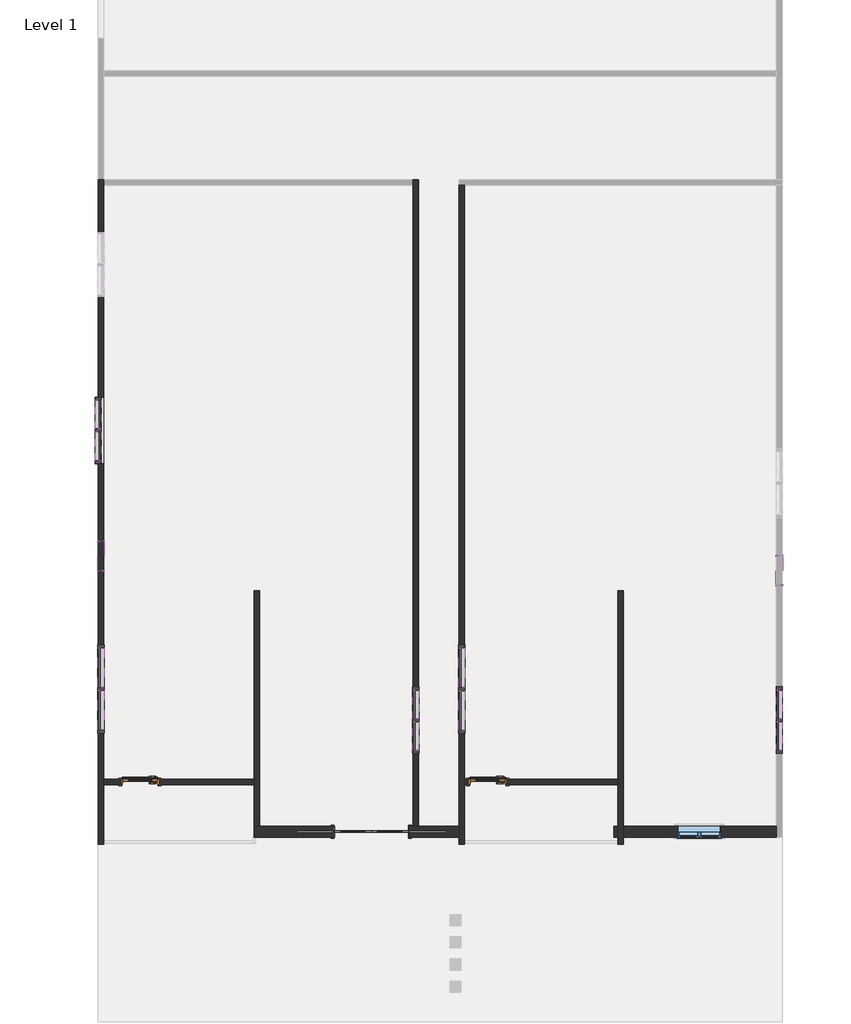
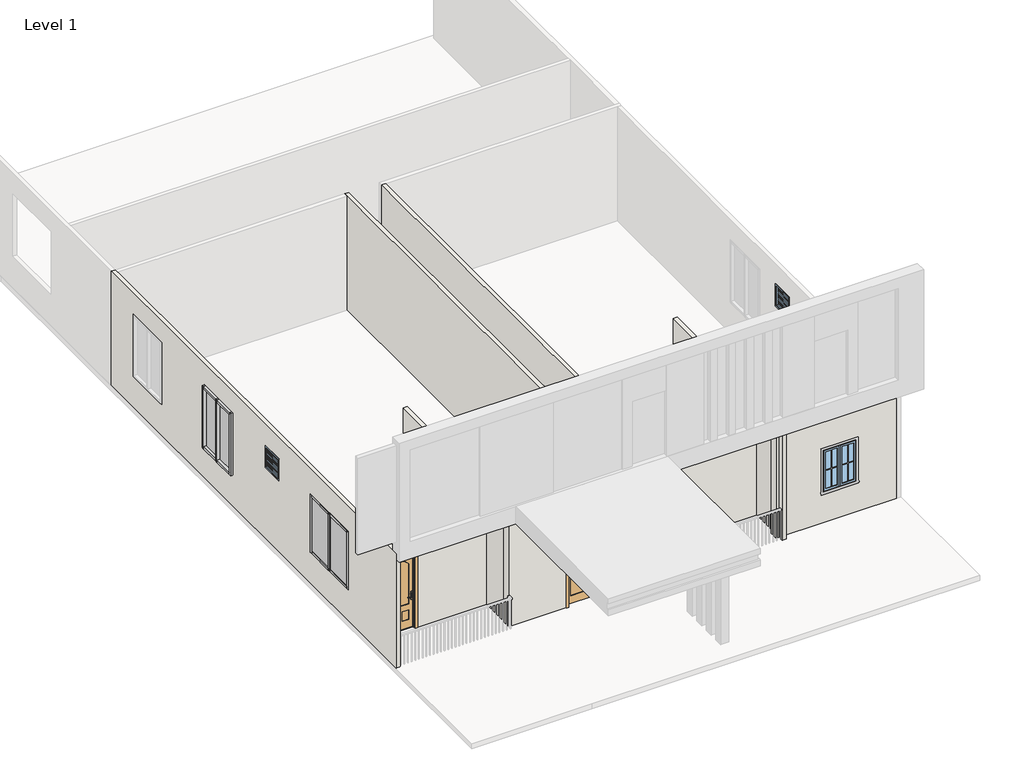
# One storey, part 1 of 3: 35 members, 10 plates, 9 walls, 3 doors, 3 windows.
"""IFC4 building model written with IfcOpenShell, lengths in millimetres."""

from ifc_helpers import new_model, si_unit, frame, origin, place, context, project, spatial, polyline, outline, extrude, faceted_brep, transform, mapped, element, save
from components import door_b81be692, door_7a66d0d1, member_8acf8d94, member_501b078b, member_2e6d4a6b, member_96ae0c19, member_d60e8053, member_2fae0574, member_b8ac15de, member_17644e48, system_panel_glazed_c4393626, system_panel_glazed_0e71bc1b, system_panel_glazed_e97abd02, system_panel_glazed_a7ecbca6, window_d341e8ac, window_d39e7ecb

model = new_model("IFC4")

# Units and contexts
model_context = context("Model", 3, world=origin())
ifc_project = project(units=[si_unit("LENGTHUNIT", "METRE", prefix="MILLI")], contexts=[model_context])

# Site, building, storey
site = spatial("IfcSite", under=ifc_project)
building = spatial("IfcBuilding", under=site)
storey = spatial("IfcBuildingStorey", under=building, Name="Level 1", Elevation=0.0)

# Doors
placement = place(None, origin())
door_shape = door_b81be692(model_context)
element("IfcDoor", 1, ObjectType="29\" x 84\"", at=placement, inside=storey, context=model_context, shape_type="MappedRepresentation", body=[
    mapped(door_shape, transform((-7346.707583, -9448.7163489, 0.0), x_axis=(1.0, 0.0, 0.0), y_axis=(0.0, 1.0, 0.0), z_axis=(0.0, 0.0, 1.0))),
])
element("IfcDoor", 2, ObjectType="29\" x 84\"", at=placement, inside=storey, context=model_context, shape_type="MappedRepresentation", body=[
    mapped(door_shape, transform((-172.2931282, -9448.9038009, 0.0), x_axis=(1.0, 0.0, 0.0), y_axis=(0.0, 1.0, 0.0), z_axis=(0.0, 0.0, 1.0))),
])
door_2_shape = door_7a66d0d1(model_context)
element("IfcDoor", 3, ObjectType="Door-Interior-Double-Pocket-2_Panel-Wood : 60\" x 84\"", at=placement, inside=storey, context=model_context, shape_type="MappedRepresentation", body=[
    mapped(door_2_shape, transform((-2570.8435762, -10471.5779557, 0.0), x_axis=(-1.0, 0.0, 0.0), y_axis=(0.0, -1.0, 0.0), z_axis=(0.0, 0.0, 1.0))),
])

# Members
member_shape = member_8acf8d94(model_context)
element("IfcMember", 4, ObjectType="Rectangular Mullion : 2.5\" x 5\" rectangular", at=placement, inside=storey, context=model_context, shape_type="MappedRepresentation", body=[
    mapped(member_shape, transform((-8153.157583, -8377.1401329, 2621.886558), x_axis=(0.0, 0.0, 1.0), y_axis=(-1.0, 0.0, 0.0), z_axis=(0.0, -1.0, 0.0))),
])
element("IfcMember", 5, ObjectType="Rectangular Mullion : 2.5\" x 5\" rectangular", at=placement, inside=storey, context=model_context, shape_type="MappedRepresentation", body=[
    mapped(member_shape, transform((-8153.157583, -7497.6651329, 2621.886558), x_axis=(0.0, 0.0, 1.0), y_axis=(-1.0, 0.0, 0.0), z_axis=(0.0, -1.0, 0.0))),
])
element("IfcMember", 6, ObjectType="Rectangular Mullion : 2.5\" x 5\" rectangular", at=placement, inside=storey, context=model_context, shape_type="MappedRepresentation", body=[
    mapped(member_shape, transform((-8153.157583, -6681.6901329, 914.4), x_axis=(0.0, 0.0, -1.0), y_axis=(-1.0, 0.0, 0.0), z_axis=(0.0, 1.0, 0.0))),
])
element("IfcMember", 7, ObjectType="Rectangular Mullion : 2.5\" x 5\" rectangular", at=placement, inside=storey, context=model_context, shape_type="MappedRepresentation", body=[
    mapped(member_shape, transform((-8153.157583, -7561.1651329, 914.4), x_axis=(0.0, 0.0, -1.0), y_axis=(-1.0, 0.0, 0.0), z_axis=(0.0, 1.0, 0.0))),
])
member_2_shape = member_501b078b(model_context)
element("IfcMember", 8, ObjectType="Rectangular Mullion : 2.5\" x 5\" rectangular", at=placement, inside=storey, context=model_context, shape_type="MappedRepresentation", body=[
    mapped(member_2_shape, transform((5848.1708786, -8795.0998253, 2743.2), x_axis=(0.0, 0.0, 1.0), y_axis=(-1.0, 0.0, 0.0), z_axis=(0.0, -1.0, 0.0))),
])
element("IfcMember", 9, ObjectType="Rectangular Mullion : 2.5\" x 5\" rectangular", at=placement, inside=storey, context=model_context, shape_type="MappedRepresentation", body=[
    mapped(member_2_shape, transform((5848.1708786, -8142.1745373, 2743.2), x_axis=(0.0, 0.0, 1.0), y_axis=(-1.0, 0.0, 0.0), z_axis=(0.0, -1.0, 0.0))),
])
element("IfcMember", 10, ObjectType="Rectangular Mullion : 2.5\" x 5\" rectangular", at=placement, inside=storey, context=model_context, shape_type="MappedRepresentation", body=[
    mapped(member_2_shape, transform((-1656.4435762, -8795.0998253, 2743.2), x_axis=(0.0, 0.0, 1.0), y_axis=(-1.0, 0.0, 0.0), z_axis=(0.0, -1.0, 0.0))),
])
element("IfcMember", 11, ObjectType="Rectangular Mullion : 2.5\" x 5\" rectangular", at=placement, inside=storey, context=model_context, shape_type="MappedRepresentation", body=[
    mapped(member_2_shape, transform((-1656.4435762, -8142.1745373, 2743.2), x_axis=(0.0, 0.0, 1.0), y_axis=(-1.0, 0.0, 0.0), z_axis=(0.0, -1.0, 0.0))),
])
element("IfcMember", 12, ObjectType="Rectangular Mullion : 2.5\" x 5\" rectangular", at=placement, inside=storey, context=model_context, shape_type="MappedRepresentation", body=[
    mapped(member_2_shape, transform((5848.1708786, -7552.7492493, 914.4), x_axis=(0.0, 0.0, -1.0), y_axis=(-1.0, 0.0, 0.0), z_axis=(0.0, 1.0, 0.0))),
])
element("IfcMember", 13, ObjectType="Rectangular Mullion : 2.5\" x 5\" rectangular", at=placement, inside=storey, context=model_context, shape_type="MappedRepresentation", body=[
    mapped(member_2_shape, transform((5848.1708786, -8205.6745373, 914.4), x_axis=(0.0, 0.0, -1.0), y_axis=(-1.0, 0.0, 0.0), z_axis=(0.0, 1.0, 0.0))),
])
element("IfcMember", 14, ObjectType="Rectangular Mullion : 2.5\" x 5\" rectangular", at=placement, inside=storey, context=model_context, shape_type="MappedRepresentation", body=[
    mapped(member_2_shape, transform((-1656.4435762, -7552.7492493, 914.4), x_axis=(0.0, 0.0, -1.0), y_axis=(-1.0, 0.0, 0.0), z_axis=(0.0, 1.0, 0.0))),
])
element("IfcMember", 15, ObjectType="Rectangular Mullion : 2.5\" x 5\" rectangular", at=placement, inside=storey, context=model_context, shape_type="MappedRepresentation", body=[
    mapped(member_2_shape, transform((-1656.4435762, -8205.6745373, 914.4), x_axis=(0.0, 0.0, -1.0), y_axis=(-1.0, 0.0, 0.0), z_axis=(0.0, 1.0, 0.0))),
])
member_3_shape = member_2e6d4a6b(model_context)
element("IfcMember", 16, ObjectType="Rectangular Mullion : 2.5\" x 5\" rectangular", at=placement, inside=storey, context=model_context, shape_type="MappedRepresentation", body=[
    mapped(member_3_shape, transform((-705.6931282, -8380.4909009, 2743.2), x_axis=(0.0, 0.0, 1.0), y_axis=(-1.0, 0.0, 0.0), z_axis=(0.0, -1.0, 0.0))),
])
element("IfcMember", 17, ObjectType="Rectangular Mullion : 2.5\" x 5\" rectangular", at=placement, inside=storey, context=model_context, shape_type="MappedRepresentation", body=[
    mapped(member_3_shape, transform((-705.6931282, -7499.3405169, 2743.2), x_axis=(0.0, 0.0, 1.0), y_axis=(-1.0, 0.0, 0.0), z_axis=(0.0, -1.0, 0.0))),
])
element("IfcMember", 18, ObjectType="Rectangular Mullion : 2.5\" x 5\" rectangular", at=placement, inside=storey, context=model_context, shape_type="MappedRepresentation", body=[
    mapped(member_3_shape, transform((-705.6931282, -6681.6901329, 914.4), x_axis=(0.0, 0.0, -1.0), y_axis=(-1.0, 0.0, 0.0), z_axis=(0.0, 1.0, 0.0))),
])
element("IfcMember", 19, ObjectType="Rectangular Mullion : 2.5\" x 5\" rectangular", at=placement, inside=storey, context=model_context, shape_type="MappedRepresentation", body=[
    mapped(member_3_shape, transform((-705.6931282, -7562.8405169, 914.4), x_axis=(0.0, 0.0, -1.0), y_axis=(-1.0, 0.0, 0.0), z_axis=(0.0, 1.0, 0.0))),
])
member_4_shape = member_96ae0c19(model_context)
element("IfcMember", 20, ObjectType="Rectangular Mullion : 2.5\" x 5\" rectangular", at=placement, inside=storey, context=model_context, shape_type="MappedRepresentation", body=[
    mapped(member_4_shape, transform((-8210.307583, -2819.4060617, 2743.2), x_axis=(0.0, 0.0, 1.0), y_axis=(-1.0, 0.0, 0.0), z_axis=(0.0, -1.0, 0.0))),
])
element("IfcMember", 21, ObjectType="Rectangular Mullion : 2.5\" x 5\" rectangular", at=placement, inside=storey, context=model_context, shape_type="MappedRepresentation", body=[
    mapped(member_4_shape, transform((-8210.307583, -2164.5788979, 2743.2), x_axis=(0.0, 0.0, 1.0), y_axis=(-1.0, 0.0, 0.0), z_axis=(0.0, -1.0, 0.0))),
])
element("IfcMember", 22, ObjectType="Rectangular Mullion : 2.5\" x 5\" rectangular", at=placement, inside=storey, context=model_context, shape_type="MappedRepresentation", body=[
    mapped(member_4_shape, transform((-8210.307583, -1573.2517341, 914.4), x_axis=(0.0, 0.0, -1.0), y_axis=(-1.0, 0.0, 0.0), z_axis=(0.0, 1.0, 0.0))),
])
element("IfcMember", 23, ObjectType="Rectangular Mullion : 2.5\" x 5\" rectangular", at=placement, inside=storey, context=model_context, shape_type="MappedRepresentation", body=[
    mapped(member_4_shape, transform((-8210.307583, -2228.0788979, 914.4), x_axis=(0.0, 0.0, -1.0), y_axis=(-1.0, 0.0, 0.0), z_axis=(0.0, 1.0, 0.0))),
])
member_5_shape = member_d60e8053(model_context)
element("IfcMember", 24, ObjectType="Rectangular Mullion : 2.5\" x 5\" rectangular", at=placement, inside=storey, context=model_context, shape_type="MappedRepresentation", body=[
    mapped(member_5_shape, transform((-8210.307583, -2196.3288979, 914.4), x_axis=(0.0, -1.0, 0.0), y_axis=(-1.0, 0.0, 0.0), z_axis=(0.0, 0.0, -1.0))),
])
member_6_shape = member_2fae0574(model_context)
element("IfcMember", 25, ObjectType="Rectangular Mullion : 2.5\" x 5\" rectangular", at=placement, inside=storey, context=model_context, shape_type="MappedRepresentation", body=[
    mapped(member_6_shape, transform((-8210.307583, -1509.7517341, 2743.2), x_axis=(0.0, 1.0, 0.0), y_axis=(-1.0, 0.0, 0.0), z_axis=(0.0, 0.0, 1.0))),
])
element("IfcMember", 26, ObjectType="Rectangular Mullion : 2.5\" x 5\" rectangular", at=placement, inside=storey, context=model_context, shape_type="MappedRepresentation", body=[
    mapped(member_6_shape, transform((-8210.307583, -2882.9060617, 914.4), x_axis=(0.0, -1.0, 0.0), y_axis=(-1.0, 0.0, 0.0), z_axis=(0.0, 0.0, -1.0))),
])
member_7_shape = member_b8ac15de(model_context)
element("IfcMember", 27, ObjectType="Rectangular Mullion : 2.5\" x 5\" rectangular", at=placement, inside=storey, context=model_context, shape_type="MappedRepresentation", body=[
    mapped(member_7_shape, transform((-8153.157583, -7529.4151329, 914.4), x_axis=(0.0, -1.0, 0.0), y_axis=(-1.0, 0.0, 0.0), z_axis=(0.0, 0.0, -1.0))),
])
member_8_shape = member_17644e48(model_context)
element("IfcMember", 28, ObjectType="Rectangular Mullion : 2.5\" x 5\" rectangular", at=placement, inside=storey, context=model_context, shape_type="MappedRepresentation", body=[
    mapped(member_8_shape, transform((-8153.157583, -6618.1901329, 2621.886558), x_axis=(0.0, 1.0, 0.0), y_axis=(-1.0, 0.0, 0.0), z_axis=(0.0, 0.0, 1.0))),
])
element("IfcMember", 29, ObjectType="Rectangular Mullion : 2.5\" x 5\" rectangular", at=placement, inside=storey, context=model_context, shape_type="MappedRepresentation", body=[
    mapped(member_8_shape, transform((-8153.157583, -8440.6401329, 914.4), x_axis=(0.0, -1.0, 0.0), y_axis=(-1.0, 0.0, 0.0), z_axis=(0.0, 0.0, -1.0))),
])
element("IfcMember", 30, ObjectType="Rectangular Mullion : 2.5\" x 5\" rectangular", at=placement, inside=storey, context=model_context, shape_type="MappedRepresentation", body=[
    mapped(member_5_shape, transform((5848.1708786, -8173.9245373, 914.4), x_axis=(0.0, -1.0, 0.0), y_axis=(-1.0, 0.0, 0.0), z_axis=(0.0, 0.0, -1.0))),
])
element("IfcMember", 31, ObjectType="Rectangular Mullion : 2.5\" x 5\" rectangular", at=placement, inside=storey, context=model_context, shape_type="MappedRepresentation", body=[
    mapped(member_5_shape, transform((-1656.4435762, -8173.9245373, 914.4), x_axis=(0.0, -1.0, 0.0), y_axis=(-1.0, 0.0, 0.0), z_axis=(0.0, 0.0, -1.0))),
])
element("IfcMember", 32, ObjectType="Rectangular Mullion : 2.5\" x 5\" rectangular", at=placement, inside=storey, context=model_context, shape_type="MappedRepresentation", body=[
    mapped(member_5_shape, transform((-705.6931282, -7531.0905169, 914.4), x_axis=(0.0, -1.0, 0.0), y_axis=(-1.0, 0.0, 0.0), z_axis=(0.0, 0.0, -1.0))),
])
element("IfcMember", 33, ObjectType="Rectangular Mullion : 2.5\" x 5\" rectangular", at=placement, inside=storey, context=model_context, shape_type="MappedRepresentation", body=[
    mapped(member_6_shape, transform((5848.1708786, -7489.2492493, 2743.2), x_axis=(0.0, 1.0, 0.0), y_axis=(-1.0, 0.0, 0.0), z_axis=(0.0, 0.0, 1.0))),
])
element("IfcMember", 34, ObjectType="Rectangular Mullion : 2.5\" x 5\" rectangular", at=placement, inside=storey, context=model_context, shape_type="MappedRepresentation", body=[
    mapped(member_6_shape, transform((-1656.4435762, -7489.2492493, 2743.2), x_axis=(0.0, 1.0, 0.0), y_axis=(-1.0, 0.0, 0.0), z_axis=(0.0, 0.0, 1.0))),
])
element("IfcMember", 35, ObjectType="Rectangular Mullion : 2.5\" x 5\" rectangular", at=placement, inside=storey, context=model_context, shape_type="MappedRepresentation", body=[
    mapped(member_6_shape, transform((-705.6931282, -6618.1901329, 2743.2), x_axis=(0.0, 1.0, 0.0), y_axis=(-1.0, 0.0, 0.0), z_axis=(0.0, 0.0, 1.0))),
])
element("IfcMember", 36, ObjectType="Rectangular Mullion : 2.5\" x 5\" rectangular", at=placement, inside=storey, context=model_context, shape_type="MappedRepresentation", body=[
    mapped(member_6_shape, transform((5848.1708786, -8858.5998253, 914.4), x_axis=(0.0, -1.0, 0.0), y_axis=(-1.0, 0.0, 0.0), z_axis=(0.0, 0.0, -1.0))),
])
element("IfcMember", 37, ObjectType="Rectangular Mullion : 2.5\" x 5\" rectangular", at=placement, inside=storey, context=model_context, shape_type="MappedRepresentation", body=[
    mapped(member_6_shape, transform((-1656.4435762, -8858.5998253, 914.4), x_axis=(0.0, -1.0, 0.0), y_axis=(-1.0, 0.0, 0.0), z_axis=(0.0, 0.0, -1.0))),
])
element("IfcMember", 38, ObjectType="Rectangular Mullion : 2.5\" x 5\" rectangular", at=placement, inside=storey, context=model_context, shape_type="MappedRepresentation", body=[
    mapped(member_6_shape, transform((-705.6931282, -8443.9909009, 914.4), x_axis=(0.0, -1.0, 0.0), y_axis=(-1.0, 0.0, 0.0), z_axis=(0.0, 0.0, -1.0))),
])

# Plates
system_panel_glazed_shape = system_panel_glazed_c4393626(model_context)
element("IfcPlate", 39, ObjectType="System Panel : Glazed", at=placement, inside=storey, context=model_context, shape_type="MappedRepresentation", body=[
    mapped(system_panel_glazed_shape, transform((-8210.307583, -1868.915316, 977.9), x_axis=(0.0, -1.0, 0.0), y_axis=(1.0, 0.0, 0.0), z_axis=(0.0, 0.0, 1.0))),
])
element("IfcPlate", 40, ObjectType="System Panel : Glazed", at=placement, inside=storey, context=model_context, shape_type="MappedRepresentation", body=[
    mapped(system_panel_glazed_shape, transform((-8210.307583, -2523.7424798, 977.9), x_axis=(0.0, -1.0, 0.0), y_axis=(1.0, 0.0, 0.0), z_axis=(0.0, 0.0, 1.0))),
])
system_panel_glazed_2_shape = system_panel_glazed_0e71bc1b(model_context)
element("IfcPlate", 41, ObjectType="System Panel : Glazed", at=placement, inside=storey, context=model_context, shape_type="MappedRepresentation", body=[
    mapped(system_panel_glazed_2_shape, transform((-8153.157583, -7089.6776329, 977.9), x_axis=(0.0, -1.0, 0.0), y_axis=(1.0, 0.0, 0.0), z_axis=(0.0, 0.0, 1.0))),
])
element("IfcPlate", 42, ObjectType="System Panel : Glazed", at=placement, inside=storey, context=model_context, shape_type="MappedRepresentation", body=[
    mapped(system_panel_glazed_2_shape, transform((-8153.157583, -7969.1526329, 977.9), x_axis=(0.0, -1.0, 0.0), y_axis=(1.0, 0.0, 0.0), z_axis=(0.0, 0.0, 1.0))),
])
system_panel_glazed_3_shape = system_panel_glazed_e97abd02(model_context)
element("IfcPlate", 43, ObjectType="System Panel : Glazed", at=placement, inside=storey, context=model_context, shape_type="MappedRepresentation", body=[
    mapped(system_panel_glazed_3_shape, transform((5848.1708786, -7847.4618933, 977.9), x_axis=(0.0, -1.0, 0.0), y_axis=(1.0, 0.0, 0.0), z_axis=(0.0, 0.0, 1.0))),
])
element("IfcPlate", 44, ObjectType="System Panel : Glazed", at=placement, inside=storey, context=model_context, shape_type="MappedRepresentation", body=[
    mapped(system_panel_glazed_3_shape, transform((-1656.4435762, -7847.4618933, 977.9), x_axis=(0.0, -1.0, 0.0), y_axis=(1.0, 0.0, 0.0), z_axis=(0.0, 0.0, 1.0))),
])
element("IfcPlate", 45, ObjectType="System Panel : Glazed", at=placement, inside=storey, context=model_context, shape_type="MappedRepresentation", body=[
    mapped(system_panel_glazed_3_shape, transform((5848.1708786, -8500.3871813, 977.9), x_axis=(0.0, -1.0, 0.0), y_axis=(1.0, 0.0, 0.0), z_axis=(0.0, 0.0, 1.0))),
])
element("IfcPlate", 46, ObjectType="System Panel : Glazed", at=placement, inside=storey, context=model_context, shape_type="MappedRepresentation", body=[
    mapped(system_panel_glazed_3_shape, transform((-1656.4435762, -8500.3871813, 977.9), x_axis=(0.0, -1.0, 0.0), y_axis=(1.0, 0.0, 0.0), z_axis=(0.0, 0.0, 1.0))),
])
system_panel_glazed_4_shape = system_panel_glazed_a7ecbca6(model_context)
element("IfcPlate", 47, ObjectType="System Panel : Glazed", at=placement, inside=storey, context=model_context, shape_type="MappedRepresentation", body=[
    mapped(system_panel_glazed_4_shape, transform((-705.6931282, -7090.5153249, 977.9), x_axis=(0.0, -1.0, 0.0), y_axis=(1.0, 0.0, 0.0), z_axis=(0.0, 0.0, 1.0))),
])
element("IfcPlate", 48, ObjectType="System Panel : Glazed", at=placement, inside=storey, context=model_context, shape_type="MappedRepresentation", body=[
    mapped(system_panel_glazed_4_shape, transform((-705.6931282, -7971.6657089, 977.9), x_axis=(0.0, -1.0, 0.0), y_axis=(1.0, 0.0, 0.0), z_axis=(0.0, 0.0, 1.0))),
])

# Walls
element("IfcWall", 49, ObjectType="4.5\" wall", at=placement, inside=storey, context=model_context, shape_type="Brep", body=[
    faceted_brep([(-8096.007583, -10738.0280197, 0.0), (-8096.007583, -9509.0413489, 0.0), (-8096.007583, -9394.7413489, 0.0), (-8096.007583, 2864.0002499, 0.0), (-8096.007583, 2978.3002499, 0.0), (-8096.007583, 2978.3002499, 3352.8), (-8096.007583, 2864.0002499, 3352.8), (-8096.007583, -9394.7413489, 3352.8), (-8096.007583, -9509.0413489, 3352.8), (-8096.007583, -10738.0280197, 3352.8), (-8096.007583, -6618.1901329, 2621.886558), (-8096.007583, -6618.1901329, 914.4), (-8096.007583, -8440.6401329, 914.4), (-8096.007583, -8440.6401329, 2621.886558), (-8096.007583, -5094.1901329, 2724.15), (-8096.007583, -4484.5901329, 2724.15), (-8096.007583, -4484.5901329, 2114.55), (-8096.007583, -5094.1901329, 2114.55), (-8096.007583, 1909.8209543, 2743.2), (-8096.007583, 1909.8209543, 914.4), (-8096.007583, 536.6666267, 914.4), (-8096.007583, 536.6666267, 2743.2), (-8096.007583, -1509.7517341, 2743.2), (-8096.007583, -1509.7517341, 914.4), (-8096.007583, -2882.9060617, 914.4), (-8096.007583, -2882.9060617, 2743.2), (-8210.307583, 2978.3002499, 0.0), (-8210.307583, -10738.0280197, 0.0), (-8210.307583, -10738.0280197, 3352.8), (-8210.307583, 2978.3002499, 3352.8), (-8210.307583, -6618.1901329, 914.4), (-8210.307583, -6618.1901329, 2621.886558), (-8210.307583, -8440.6401329, 2621.886558), (-8210.307583, -8440.6401329, 914.4), (-8210.307583, -5094.1901329, 2724.15), (-8210.307583, -5094.1901329, 2114.55), (-8210.307583, -4484.5901329, 2114.55), (-8210.307583, -4484.5901329, 2724.15), (-8210.307583, 1909.8209543, 914.4), (-8210.307583, 1909.8209543, 2743.2), (-8210.307583, 536.6666267, 2743.2), (-8210.307583, 536.6666267, 914.4), (-8210.307583, -1509.7517341, 914.4), (-8210.307583, -1509.7517341, 2743.2), (-8210.307583, -2882.9060617, 2743.2), (-8210.307583, -2882.9060617, 914.4)], [[[0, 1, 2, 3, 4, 5, 6, 7, 8, 9], [10, 11, 12, 13], [14, 15, 16, 17], [18, 19, 20, 21], [22, 23, 24, 25]], [[26, 27, 28, 29], [30, 31, 32, 33], [34, 35, 36, 37], [38, 39, 40, 41], [42, 43, 44, 45]], [[4, 3, 2, 1, 0, 27, 26]], [[9, 8, 7, 6, 5, 29, 28]], [[0, 9, 28, 27]], [[5, 4, 26, 29]], [[10, 31, 30, 11]], [[31, 10, 13, 32]], [[32, 13, 12, 33]], [[11, 30, 33, 12]], [[35, 34, 14, 17]], [[36, 35, 17, 16]], [[37, 36, 16, 15]], [[34, 37, 15, 14]], [[38, 19, 18, 39]], [[39, 18, 21, 40]], [[40, 21, 20, 41]], [[19, 38, 41, 20]], [[22, 43, 42, 23]], [[43, 22, 25, 44]], [[44, 25, 24, 45]], [[23, 42, 45, 24]]]),
])
element("IfcWall", 50, ObjectType="4.5\" wall", at=placement, inside=storey, context=model_context, shape_type="Brep", body=[
    faceted_brep([(-1599.2935762, -10357.2779557, 0.0), (-1599.2935762, 2978.3002499, 0.0), (-1599.2935762, 2978.3002499, 3352.8), (-1599.2935762, -10357.2779557, 3352.8), (-1599.2935762, -7489.2492493, 2743.2), (-1599.2935762, -7489.2492493, 914.4), (-1599.2935762, -8858.5998253, 914.4), (-1599.2935762, -8858.5998253, 2743.2), (-1713.5935762, 2978.3002499, 0.0), (-1713.5935762, 2864.0002499, 0.0), (-1713.5935762, -10357.2779557, 0.0), (-1713.5935762, -10357.2779557, 3352.8), (-1713.5935762, 2864.0002499, 3352.8), (-1713.5935762, 2978.3002499, 3352.8), (-1713.5935762, -7489.2492493, 914.4), (-1713.5935762, -7489.2492493, 2743.2), (-1713.5935762, -8858.5998253, 2743.2), (-1713.5935762, -8858.5998253, 914.4)], [[[0, 1, 2, 3], [4, 5, 6, 7]], [[8, 9, 10, 11, 12, 13], [14, 15, 16, 17]], [[1, 0, 10, 9, 8]], [[3, 2, 13, 12, 11]], [[2, 1, 8, 13]], [[0, 3, 11, 10]], [[14, 5, 4, 15]], [[15, 4, 7, 16]], [[16, 7, 6, 17]], [[5, 14, 17, 6]]]),
])
element("IfcWall", 51, ObjectType="4.5\" wall", at=placement, inside=storey, context=model_context, shape_type="Brep", body=[
    faceted_brep([(-762.8431282, 2864.0002499, 0.0), (-762.8431282, -10357.2779557, 0.0), (-762.8431282, -10450.9404557, 0.0), (-762.8431282, -10492.2154557, 0.0), (-762.8431282, -10585.8779557, 0.0), (-762.8431282, -10737.6531157, 0.0), (-762.8431282, -10737.6531157, 3352.8), (-762.8431282, -10585.8779557, 3352.8), (-762.8431282, -10357.2779557, 3352.8), (-762.8431282, 2864.0002499, 3352.8), (-762.8431282, -6618.1901329, 914.4), (-762.8431282, -6618.1901329, 2743.2), (-762.8431282, -8443.9909009, 2743.2), (-762.8431282, -8443.9909009, 914.4), (-648.5431282, -10737.6531157, 0.0), (-648.5431282, -9509.2288009, 0.0), (-648.5431282, -9394.9288009, 0.0), (-648.5431282, 2864.0002499, 0.0), (-648.5431282, 2864.0002499, 3352.8), (-648.5431282, -9394.9288009, 3352.8), (-648.5431282, -9509.2288009, 3352.8), (-648.5431282, -10737.6531157, 3352.8), (-648.5431282, -6618.1901329, 2743.2), (-648.5431282, -6618.1901329, 914.4), (-648.5431282, -8443.9909009, 914.4), (-648.5431282, -8443.9909009, 2743.2)], [[[0, 1, 2, 3, 4, 5, 6, 7, 8, 9], [10, 11, 12, 13]], [[14, 15, 16, 17, 18, 19, 20, 21], [22, 23, 24, 25]], [[5, 4, 3, 2, 1, 0, 17, 16, 15, 14]], [[6, 5, 14, 21]], [[9, 8, 7, 6, 21, 20, 19, 18]], [[0, 9, 18, 17]], [[10, 23, 22, 11]], [[11, 22, 25, 12]], [[12, 25, 24, 13]], [[23, 10, 13, 24]]]),
])
element("IfcWall", 52, ObjectType="4.5\" wall", at=placement, inside=storey, context=model_context, shape_type="Brep", body=[
    faceted_brep([(-4874.3237038, -10357.2779557, 0.0), (-4874.3237038, -5507.4946657, 0.0), (-4874.3237038, -5507.4946657, 3352.8), (-4874.3237038, -10357.2779557, 3352.8), (-4988.6237038, -10357.2779557, 0.0), (-4988.6237038, -10357.2779557, 3352.8), (-4988.6237038, -9509.0413489, 3352.8), (-4988.6237038, -9394.7413489, 3352.8), (-4988.6237038, -5507.4946657, 3352.8), (-4988.6237038, -5507.4946657, 0.0), (-4988.6237038, -9394.7413489, 0.0), (-4988.6237038, -9509.0413489, 0.0)], [[[0, 1, 2, 3]], [[4, 5, 6, 7, 8, 9, 10, 11]], [[1, 0, 4, 11, 10, 9]], [[2, 1, 9, 8]], [[3, 2, 8, 7, 6, 5]], [[0, 3, 5, 4]]]),
])
element("IfcWall", 53, ObjectType="4.5\" wall", at=placement, inside=storey, context=model_context, shape_type="Brep", body=[
    faceted_brep([(2515.990751, -5507.4946657, 0.0), (2515.990751, -9394.9288009, 0.0), (2515.990751, -9509.2288009, 0.0), (2515.990751, -10737.6531157, 0.0), (2515.990751, -10737.6531157, 3352.8), (2515.990751, -9509.2288009, 3352.8), (2515.990751, -9394.9288009, 3352.8), (2515.990751, -5507.4946657, 3352.8), (2630.290751, -5507.4946657, 0.0), (2630.290751, -5507.4946657, 3352.8), (2630.290751, -10737.6531157, 3352.8), (2630.290751, -10737.6531157, 0.0)], [[[0, 1, 2, 3, 4, 5, 6, 7]], [[8, 9, 10, 11]], [[3, 2, 1, 0, 8, 11]], [[4, 3, 11, 10]], [[7, 6, 5, 4, 10, 9]], [[0, 7, 9, 8]]]),
])
element("IfcWall", 54, ObjectType="4.5\" wall", at=placement, inside=storey, context=model_context, shape_type="SweptSolid", body=[
    extrude(outline(polyline([(3352.8, -4988.6237038), (3352.8, -8096.007583), (0.0, -8096.007583), (0.0, -7740.407583), (2159.0, -7740.407583), (2159.0, -6953.007583), (0.0, -6953.007583), (0.0, -4988.6237038), (3352.8, -4988.6237038)])), frame((0.0, -9509.0413489, 0.0), z_axis=(0.0, 1.0, 0.0), x_axis=(0.0, 0.0, 1.0)), (0.0, 0.0, 1.0), 114.3),
])
element("IfcWall", 55, ObjectType="4.5\" wall", at=placement, inside=storey, context=model_context, shape_type="SweptSolid", body=[
    extrude(outline(polyline([(3352.8, 2515.990751), (3352.8, -648.5431282), (0.0, -648.5431282), (0.0, -565.9931282), (2159.0, -565.9931282), (2159.0, 221.4068718), (0.0, 221.4068718), (0.0, 2515.990751), (3352.8, 2515.990751)])), frame((0.0, -9509.2288009, 0.0), z_axis=(0.0, 1.0, 0.0), x_axis=(0.0, 0.0, 1.0)), (0.0, 0.0, 1.0), 114.3),
])
element("IfcWall", 56, ObjectType="9\" wall", at=placement, inside=storey, context=model_context, shape_type="Brep", body=[
    faceted_brep([(-4996.231207, -10357.2779557, 0.0), (-4996.231207, -10357.2779557, 3352.8), (-4988.6237038, -10357.2779557, 3352.8), (-4874.3237038, -10357.2779557, 3352.8), (-1713.5935762, -10357.2779557, 3352.8), (-1599.2935762, -10357.2779557, 3352.8), (-762.8431282, -10357.2779557, 3352.8), (-762.8431282, -10357.2779557, 0.0), (-1599.2935762, -10357.2779557, 0.0), (-1713.5935762, -10357.2779557, 0.0), (-1783.4435762, -10357.2779557, 0.0), (-1783.4435762, -10357.2779557, 2159.0), (-3358.2435762, -10357.2779557, 2159.0), (-3358.2435762, -10357.2779557, 0.0), (-4874.3237038, -10357.2779557, 0.0), (-4988.6237038, -10357.2779557, 0.0), (-4996.231207, -10585.8779557, 3352.8), (-4996.231207, -10585.8779557, 0.0), (-3358.2435762, -10585.8779557, 0.0), (-3358.2435762, -10585.8779557, 2159.0), (-1783.4435762, -10585.8779557, 2159.0), (-1783.4435762, -10585.8779557, 0.0), (-762.8431282, -10585.8779557, 0.0), (-762.8431282, -10585.8779557, 3352.8), (-3358.2435762, -10450.9404557, 0.0), (-4120.2435762, -10450.9404557, 0.0), (-4120.2435762, -10492.2154557, 0.0), (-3358.2435762, -10492.2154557, 0.0), (-1783.4435762, -10492.2154557, 0.0), (-1021.4435762, -10492.2154557, 0.0), (-1021.4435762, -10450.9404557, 0.0), (-1783.4435762, -10450.9404557, 0.0), (-4120.2435762, -10492.2154557, 2159.0), (-4120.2435762, -10450.9404557, 2159.0), (-3358.2435762, -10450.9404557, 2159.0), (-1783.4435762, -10450.9404557, 2159.0), (-1021.4435762, -10450.9404557, 2159.0), (-1021.4435762, -10492.2154557, 2159.0), (-1783.4435762, -10492.2154557, 2159.0), (-3358.2435762, -10492.2154557, 2159.0)], [[[0, 1, 2, 3, 4, 5, 6, 7, 8, 9, 10, 11, 12, 13, 14, 15]], [[16, 17, 18, 19, 20, 21, 22, 23]], [[17, 0, 15, 14, 13, 24, 25, 26, 27, 18]], [[7, 22, 21, 28, 29, 30, 31, 10, 9, 8]], [[1, 0, 17, 16]], [[6, 5, 4, 3, 2, 1, 16, 23]], [[7, 6, 23, 22]], [[32, 33, 34, 12, 11, 35, 36, 37, 38, 20, 19, 39]], [[32, 39, 27, 26]], [[39, 19, 18, 27]], [[20, 38, 28, 21]], [[38, 37, 29, 28]], [[37, 36, 30, 29]], [[36, 35, 31, 30]], [[35, 11, 10, 31]], [[12, 34, 24, 13]], [[34, 33, 25, 24]], [[33, 32, 26, 25]]]),
])
element("IfcWall", 57, ObjectType="9\" wall", at=placement, inside=storey, context=model_context, shape_type="SweptSolid", body=[
    extrude(outline(polyline([(0.0, 5791.0208786), (3352.8, 5791.0208786), (3352.8, 2436.2994194), (0.0, 2436.2994194), (0.0, 5791.0208786)]), holes=[polyline([(2133.6, 3739.9708786), (2133.6, 4654.3708786), (914.4, 4654.3708786), (914.4, 3739.9708786), (2133.6, 3739.9708786)])]), frame((0.0, -10585.8779557, 0.0), z_axis=(0.0, 1.0, 0.0), x_axis=(0.0, 0.0, 1.0)), (0.0, 0.0, 1.0), 228.6),
])

# Windows
window_shape = window_d341e8ac(model_context)
element("IfcWindow", 58, ObjectType="Window-Casement-Double : 36\" x 48\"", at=placement, inside=storey, context=model_context, shape_type="MappedRepresentation", body=[
    mapped(window_shape, transform((4197.1708786, -10471.5779557, 0.0), x_axis=(-1.0, 0.0, 0.0), y_axis=(0.0, -1.0, 0.0), z_axis=(0.0, 0.0, 1.0))),
])
window_2_shape = window_d39e7ecb(model_context)
element("IfcWindow", 59, ObjectType="Window-Louvers : 24\" x 24\"", at=placement, inside=storey, context=model_context, shape_type="MappedRepresentation", body=[
    mapped(window_2_shape, transform((-8159.507583, -4789.3901329, 1200.15), x_axis=(0.0, 1.0, 0.0), y_axis=(-1.0, 0.0, 0.0), z_axis=(0.0, 0.0, 1.0))),
])
element("IfcWindow", 60, ObjectType="Window-Louvers : 24\" x 24\"", at=placement, inside=storey, context=model_context, shape_type="MappedRepresentation", body=[
    mapped(window_2_shape, transform((5854.5208786, -5089.4021821, 1238.25), x_axis=(0.0, -1.0, 0.0), y_axis=(1.0, 0.0, 0.0), z_axis=(0.0, 0.0, 1.0))),
])

save(model, "model.ifc")

# Revit data of these elements
# Type "29\" x 84\""
#   Type Mark = "8"
#   Assembly Code = "B2030100"
#   Analytic Construction = "French door, wood frame with single glass"
#   Threshold Offset [instance default] = 0' - 0 1/2"
#   Thickness = 0' - 1 3/8"
#   Thermal Resistance (R) = 1.0696 (h·ft²·°F)/BTU
#   Swing Angle [instance default] = 90.00°
#   Stiles = 0' - 4 3/4"
#   Rough Width = 2' - 7"
#   Rough Height = 7' - 1"
#   Radius = 1' - 0.00625"
#   Lock Rail = 0' - 7 1/8"
#   Height = 7' - 0"
#   Width = 2' - 5"
#   Heat Transfer Coefficient (U) = 0.9350 BTU/(h·ft²·°F)
#   Door Offset [instance default] = 0' - 0"
#   Bottom Rail = 0' - 9 1/2"
#   Threshold [instance default] = yes
#   Function = 1
#   Exterior Trim [instance default] = yes
#   Trim Material = Cherry
#   Threshold Material = Cherry
#   Panel Material = Cherry
#   Glazing = Glass
#   Frame Material = Cherry
#   Door Handle Material = Aluminum
#   Visual Light Transmittance = 0
#   Solar Heat Gain Coefficient = 0
#   Wall Closure = (empty or 0)
#   Construction Type = (empty or 0)
# Type "Door-Interior-Double-Pocket-2_Panel-Wood : 60\" x 84\""
#   Type Mark = "9"
#   Assembly Code = "C1020300"
#   Analytic Construction = "Wooden"
#   Top Rail = 0' - 4 11/16"
#   Thickness = 0' - 1 3/8"
#   Thermal Resistance (R) = 2.5876 (h·ft²·°F)/BTU
#   Stiles = 0' - 4 3/4"
#   Rough Width = 10' - 2"
#   Rough Height = 7' - 4 1/2"
#   Panel Width = 2' - 6"
#   Lock Rail = 0' - 7 1/2"
#   Location [instance default] = 2' - 7"
#   Height = 7' - 0"
#   Width = 5' - 0"
#   Heat Transfer Coefficient (U) = 0.3865 BTU/(h·ft²·°F)
#   Bottom Rail = 0' - 9 1/8"
#   Panel Open [instance default] = no
#   Trim Material = Cherry
#   Panel Material = Cherry
#   Frame Material = Cherry
#   Visual Light Transmittance = 0
#   Solar Heat Gain Coefficient = 0
#   Wall Closure = (empty or 0)
#   Function = (empty or 0)
# Type "Rectangular Mullion : 2.5\" x 5\" rectangular"
#   built-in parameter 1007304 = 0.416667 (stored number, unit not read)
#   built-in parameter 1007301 = 0.104167 (stored number, unit not read)
#   built-in parameter 1007300 = 0.104167 (stored number, unit not read)
# Type "System Panel : Glazed"
#   Construction Type Id = "GSP4R"
#   Analytic Construction = "1/8 in Pilkington single glazing"
#   Visual Light Transmittance = 0.9
#   Solar Heat Gain Coefficient = 0.86
#   Heat Transfer Coefficient (U) = 1.18115 BTU/(h·ft²·°F)
#   Define Thermal Properties by = 1
# Type "4.5\" wall"
#   Assembly Code = "B2010"
#   Layers, outside or top first: 0' - 4 1/2" no material (function 1)
# Type "9\" wall"
#   Assembly Code = "B2010"
#   Layers, outside or top first: 0' - 9" no material (function 1)
# Type "Window-Casement-Double : 36\" x 48\""
#   Type Mark = "14"
#   Fire Rating = "0.5h"
#   Assembly Code = "B2020100"
#   Analytic Construction = "Double glazing - domestic"
#   Frame Extension [instance default] = 0' - 0 1/4"
#   Window Inset [instance default] = 0' - 0"
#   Wall Thickness [instance default] = 0' - 6"
#   Interior Wall Closure [instance default] = 0' - 2 1/4"
#   Half Width = 1' - 6"
#   Visual Light Transmittance = 0.81
#   Thermal Resistance (R) = 1.8146 (h·ft²·°F)/BTU
#   Solar Heat Gain Coefficient = 0.76
#   Rough Width = 3' - 0 1/2"
#   Rough Height = 4' - 0 1/2"
#   Height = 4' - 0"
#   Heat Transfer Coefficient (U) = 0.5511 BTU/(h·ft²·°F)
#   Exterior Wall Closure [instance default] = 0' - 1 1/4"
#   Extension Jamb [instance default] = 0' - 2 1/4"
#   Default Sill Height = 3' - 0"
#   Width = 3' - 0"
#   Define Thermal Properties by = 0
#   Muntin Visibility = yes
#   Interior Trim Visibility [instance default] = yes
#   Exterior Trim Visibility [instance default] = yes
#   Extension Jamb Visibility [instance default] = yes
#   Interior Trim Material = Wood - Stained
#   Muntin Pattern = Muntin Pattern_2x2 : Muntin Pattern_2x2
#   Interior Trim = Trim-Window-Interior-Flat : Picture Frame
#   Interior Frame Material = Wood - Stained
#   Glass Panel Material = Glass
#   Exterior Trim Material = Clad - White
#   Exterior Trim = Trim-Window-Exterior-Flat : with Sill
#   Exterior Frame Material = Clad - White
#   Wall Closure = (empty or 0)
# Type "Window-Louvers : 24\" x 24\""
#   Type Mark = "18"
#   Construction Type Id = "GSP4R"
#   Assembly Code = "B20"
#   Analytic Construction = "1/8 in Pilkington single glazing"
#   Visual Light Transmittance = 0.9
#   Thermal Resistance (R) = 1.53941 (h·ft²·°F)/BTU
#   Solar Heat Gain Coefficient = 0.78
#   Max Height = 1' - 11.74264"
#   Height = 2' - 0"
#   Heat Transfer Coefficient (U) = 0.6496 BTU/(h·ft²·°F)
#   Blade Width [instance default] = 1' - 10 1/2"
#   Blade Vertical Thickness = 0' - 0.35355"
#   Blade Thickness = 0' - 0 1/4"
#   Blade Spacing = 0' - 1 1/2"
#   Blade Height = 0' - 1.85355"
#   Blade Depth = 0' - 3"
#   Blade Angle = 45.00°
#   Default Sill Height = 3' - 0"
#   Trim Projection_Exterior = 0' - 0 1/2"
#   Trim Projection_Interior = 0' - 0 1/2"
#   Trim Width_Exterior = 0' - 1 1/2"
#   Trim Width_Interior = 0' - 1 1/2"
#   Width = 2' - 0"
#   Max Blade Count = 12
#   Define Thermal Properties by = 1
#   Blade Count = 12
#   Frame Material = Birch
#   Louver Material = Birch
#   Trim Exterior Material = Birch
#   Trim Interior Material = Birch
#   Wall Closure = (empty or 0)
# Elements 1, 2 (IfcDoor, "29\" x 84\"")
#   Threshold Offset = 0' - 0 1/2"
#   Swing Angle = 90.00°
#   Door Offset = 0' - 0"
#   Threshold = yes
#   Exterior Trim = yes
#   Phase Created = New Construction
#   Materials on its faces: "Cherry", "Aluminum", "Glass"
# Element 3 (IfcDoor, "Door-Interior-Double-Pocket-2_Panel-Wood : 60\" x 84\"")
#   Location = 2' - 7"
#   Panel Open = no
#   Phase Created = New Construction
#   Materials on its faces: "Cherry"
# Elements 4, 5, 6, 7, 8, 9, 10, 11, 12, 13, 14, 15, 16, 17, 18, 19, 20, 21, 22, 23, 24, 25, 26, 27, 28, 29, 30, 31, 32, 33, 34, 35, 36, 37, 38 (IfcMember, "Rectangular Mullion : 2.5\" x 5\" rectangular")
#   Phase Created = New Construction
#   Materials on its faces: "Aluminum"
# Elements 39, 40, 41, 42, 43, 44, 45, 46, 47, 48 (IfcPlate, "System Panel : Glazed")
#   Phase Created = New Construction
#   Materials on its faces: "Glass"
# Elements 49, 50, 51, 52, 53, 54, 55 (IfcWall, "4.5\" wall")
#   Top Offset = 0' - 0"
#   Base Offset = 0' - 0"
#   wall height = 11' - 0"
#   Phase Created = New Construction
#   Base Constraint = Level 1
#   Top Constraint = Level 2
#   Materials on its faces: "Default Wall"
# Elements 56, 57 (IfcWall, "9\" wall")
#   Top Offset = 0' - 0"
#   Base Offset = 0' - 0"
#   wall height = 11' - 0"
#   Phase Created = New Construction
#   Base Constraint = Level 1
#   Top Constraint = Level 2
#   Materials on its faces: "Default Wall"
# Element 58 (IfcWindow, "Window-Casement-Double : 36\" x 48\"")
#   Mark = "2"
#   Window Inset = 0' - 0"
#   Interior Wall Closure = 0' - 2 1/4"
#   Frame Extension = 0' - 0 1/4"
#   Exterior Wall Closure = 0' - 1 1/4"
#   Interior Trim Visibility = yes
#   Exterior Trim Visibility = yes
#   Phase Created = New Construction
#   Materials on its faces: "Wood - Stained", "Glass", "Clad - White"
# Element 59 (IfcWindow, "Window-Louvers : 24\" x 24\"")
#   Mark = "3"
#   Blade Width = 1' - 10 1/2"
#   Phase Created = New Construction
#   Materials on its faces: "Birch"
# Element 60 (IfcWindow, "Window-Louvers : 24\" x 24\"")
#   Mark = "4"
#   Blade Width = 1' - 10 1/2"
#   Phase Created = New Construction
#   Materials on its faces: "Birch"
# Materials
#   "Cherry": class "Wood", colour RGB 226 177 128, transparency 0, Description = "Prunus Serotina", Cost = 0
#   "Glass": class "Glass", colour RGB 0 128 192, transparency 0.75, Description = "Soda Lime Glass", Cost = 0
#   "Aluminum": class "Metal", colour RGB 247 247 247, transparency 0, Description = "Aluminum 6061", Cost = 0
#   "Wood - Stained": class "Wood", colour RGB 224 178 126, transparency 0, Cost = 0
#   "Clad - White": class "Wood", colour RGB 242 242 238, transparency 0, Cost = 0
#   "Birch": class "Wood", colour RGB 224 178 126, transparency 0, Description = "Betula Alleghaniensis", Cost = 0
#   "Default Wall": colour RGB 128 128 128, transparency 0, Cost = 0
